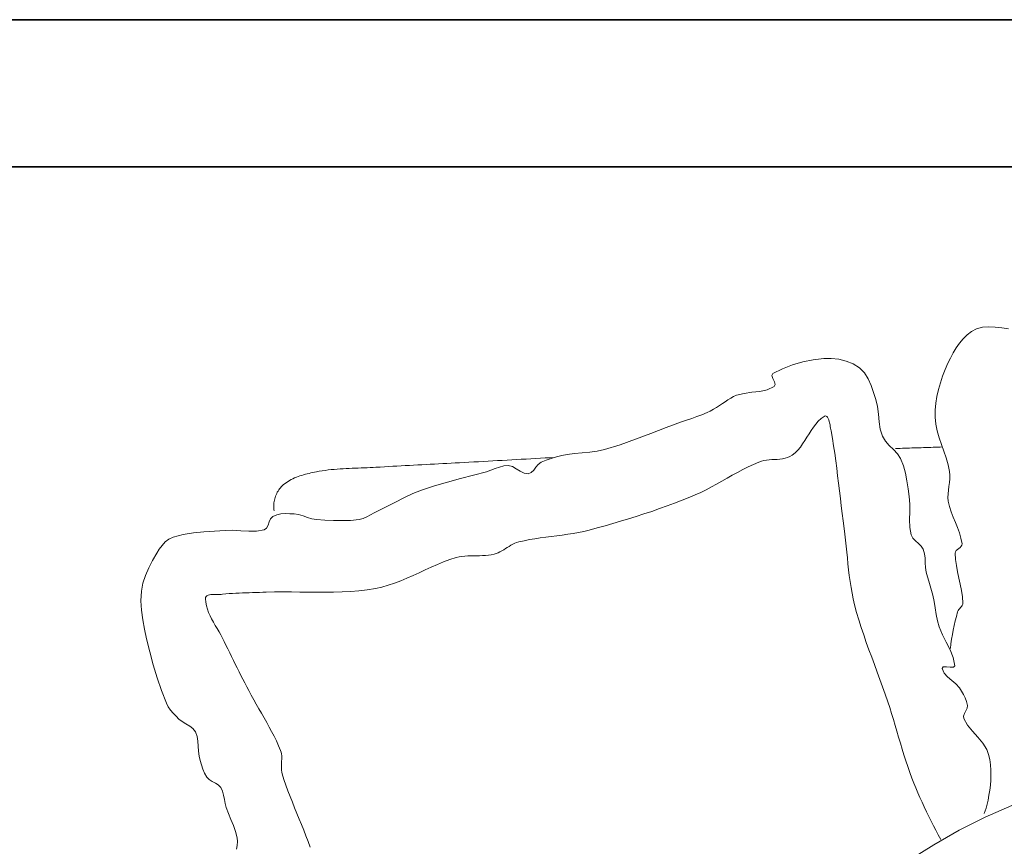
# Model space of a CAD drawing. Units: inches. Extents: x -36302355 to 648, y -221479757 to 75.
# Tile 26 of 37: x 190 to 220, y -192 to -167. Entities that reach past the tile are written whole.
import ezdxf

# ---------------------------------------------------------------- set-up
doc = ezdxf.new("R2010")
doc.units = ezdxf.units.IN
doc.header["$MEASUREMENT"] = 0
doc.layers.add('A-FURN', color=8, linetype='Continuous', lineweight=13)
doc.layers.add('A-WALL', color=7, linetype='Continuous', lineweight=35)

# ---------------------------------------------------------------- blocks, each defined once
blk = doc.blocks.new('BED-DOUBLE')
for p, q in [((26.757, 79.348), (26.607, 79.27)), ((26.943, 79.401), (26.757, 79.348)), ((27.135, 79.418), (26.943, 79.401)), ((27.332, 79.407), (27.135, 79.418)), ((27.532, 79.381), (27.332, 79.407)), ((27.733, 79.348), (27.532, 79.381)), ((26.347, 79.049), (26.235, 78.914)), ((26.471, 79.169), (26.347, 79.049)), ((26.607, 79.27), (26.471, 79.169)), ((26.134, 78.768), (26.042, 78.615)), ((26.235, 78.914), (26.134, 78.768)), ((21.435, 78.344), (21.756, 78.407)), ((21.756, 78.407), (22.08, 78.443)), ((22.08, 78.443), (22.309, 78.445)), ((22.309, 78.445), (22.541, 78.42)), ((22.541, 78.42), (22.768, 78.366)), ((25.959, 78.459), (25.883, 78.303)), ((26.042, 78.615), (25.959, 78.459)), ((20.524, 77.986), (20.815, 78.133)), ((20.815, 78.133), (21.12, 78.252)), ((21.12, 78.252), (21.435, 78.344)), ((22.768, 78.366), (22.981, 78.28)), ((22.981, 78.28), (23.172, 78.159)), ((23.172, 78.159), (23.323, 78.006)), ((25.797, 78.108), (25.719, 77.908)), ((25.883, 78.303), (25.797, 78.108)), ((20.495, 77.926), (20.524, 77.986)), ((20.521, 77.836), (20.495, 77.926)), ((20.567, 77.736), (20.521, 77.836)), ((23.323, 78.006), (23.44, 77.822)), ((23.44, 77.822), (23.532, 77.618)), ((25.719, 77.908), (25.65, 77.704)), ((20.119, 77.44), (20.35, 77.491)), ((20.35, 77.491), (20.565, 77.584)), ((20.565, 77.584), (20.594, 77.646)), ((20.594, 77.646), (20.567, 77.736)), ((23.532, 77.618), (23.607, 77.405)), ((25.593, 77.496), (25.546, 77.286)), ((25.65, 77.704), (25.593, 77.496)), ((19.065, 77.119), (19.147, 77.177)), ((19.147, 77.177), (19.23, 77.234)), ((19.23, 77.234), (19.317, 77.284)), ((19.317, 77.284), (19.408, 77.323)), ((19.408, 77.323), (19.64, 77.378)), ((19.64, 77.378), (19.88, 77.41)), ((19.88, 77.41), (20.119, 77.44)), ((23.607, 77.405), (23.677, 77.194)), ((23.677, 77.194), (23.73, 76.972)), ((25.546, 77.286), (25.513, 77.074)), ((18.605, 76.837), (18.7, 76.891)), ((18.7, 76.891), (18.794, 76.949)), ((18.794, 76.949), (18.887, 77.007)), ((18.887, 77.007), (18.98, 77.065)), ((18.98, 77.065), (19.065, 77.119)), ((23.73, 76.972), (23.756, 76.743)), ((25.513, 77.074), (25.494, 76.862)), ((17.88, 76.561), (18.038, 76.614)), ((18.038, 76.614), (18.196, 76.668)), ((18.196, 76.668), (18.352, 76.726)), ((18.352, 76.726), (18.506, 76.789)), ((18.506, 76.789), (18.605, 76.837)), ((21.911, 76.527), (21.997, 76.607)), ((21.997, 76.607), (22.092, 76.675)), ((22.092, 76.675), (22.122, 76.687)), ((22.122, 76.687), (22.15, 76.685)), ((22.15, 76.685), (22.174, 76.67)), ((22.174, 76.67), (22.196, 76.645)), ((22.196, 76.645), (22.215, 76.61)), ((22.215, 76.61), (22.232, 76.569)), ((22.232, 76.569), (22.247, 76.522)), ((23.756, 76.743), (23.776, 76.512)), ((25.494, 76.862), (25.489, 76.649)), ((25.489, 76.649), (25.507, 76.436)), ((16.786, 76.152), (17.253, 76.332)), ((17.253, 76.332), (17.722, 76.507)), ((17.722, 76.507), (17.88, 76.561)), ((21.693, 76.245), (21.761, 76.345)), ((21.761, 76.345), (21.833, 76.44)), ((21.833, 76.44), (21.911, 76.527)), ((22.247, 76.522), (22.26, 76.472)), ((22.26, 76.472), (22.271, 76.419)), ((22.271, 76.419), (22.281, 76.367)), ((22.281, 76.367), (22.29, 76.317)), ((22.29, 76.317), (22.297, 76.271)), ((22.297, 76.271), (22.304, 76.23)), ((23.776, 76.512), (23.809, 76.285)), ((23.809, 76.285), (23.875, 76.067)), ((25.507, 76.436), (25.55, 76.227)), ((15.847, 75.807), (16.318, 75.975)), ((16.318, 75.975), (16.786, 76.152)), ((21.5, 75.934), (21.565, 76.038)), ((21.565, 76.038), (21.628, 76.142)), ((21.628, 76.142), (21.693, 76.245)), ((22.304, 76.23), (22.343, 76.002)), ((22.343, 76.002), (22.38, 75.774)), ((23.875, 76.067), (23.965, 75.917)), ((25.55, 76.227), (25.61, 76.02)), ((25.61, 76.02), (25.681, 75.814)), ((15.37, 75.658), (15.847, 75.807)), ((21.288, 75.644), (21.364, 75.736)), ((21.364, 75.736), (21.434, 75.833)), ((21.434, 75.833), (21.5, 75.934)), ((22.38, 75.774), (22.414, 75.545)), ((23.965, 75.917), (24.086, 75.786)), ((24.086, 75.786), (24.218, 75.662)), ((24.218, 75.662), (24.341, 75.531)), ((24.272, 75.689), (24.344, 75.691)), ((24.344, 75.691), (24.416, 75.694)), ((24.416, 75.694), (24.488, 75.697)), ((24.488, 75.697), (24.56, 75.699)), ((24.56, 75.699), (24.632, 75.702)), ((24.632, 75.702), (24.704, 75.704)), ((24.704, 75.704), (24.776, 75.707)), ((24.776, 75.707), (24.848, 75.709)), ((24.848, 75.709), (24.92, 75.712)), ((24.92, 75.712), (24.992, 75.714)), ((24.992, 75.714), (25.064, 75.717)), ((25.064, 75.717), (25.136, 75.719)), ((25.136, 75.719), (25.208, 75.722)), ((25.208, 75.722), (25.28, 75.724)), ((25.28, 75.724), (25.353, 75.727)), ((25.353, 75.727), (25.425, 75.729)), ((25.425, 75.729), (25.497, 75.732)), ((25.497, 75.732), (25.569, 75.734)), ((25.569, 75.734), (25.641, 75.737)), ((25.641, 75.737), (25.713, 75.74)), ((25.681, 75.814), (25.756, 75.609)), ((12.675, 75.353), (12.821, 75.362)), ((12.821, 75.362), (12.966, 75.37)), ((12.966, 75.37), (13.112, 75.378)), ((13.112, 75.378), (13.258, 75.386)), ((13.258, 75.386), (13.403, 75.395)), ((13.403, 75.395), (13.549, 75.403)), ((13.549, 75.403), (13.694, 75.411)), ((13.578, 75.336), (13.736, 75.39)), ((13.694, 75.411), (13.84, 75.419)), ((13.736, 75.39), (13.898, 75.435)), ((13.898, 75.435), (14.062, 75.473)), ((14.062, 75.473), (14.226, 75.506)), ((14.226, 75.506), (14.454, 75.541)), ((14.454, 75.541), (14.685, 75.562)), ((14.685, 75.562), (14.916, 75.581)), ((14.916, 75.581), (15.145, 75.609)), ((15.145, 75.609), (15.37, 75.658)), ((20.576, 75.355), (20.658, 75.36)), ((20.658, 75.36), (20.74, 75.367)), ((20.74, 75.367), (20.82, 75.378)), ((20.82, 75.378), (20.898, 75.394)), ((20.898, 75.394), (20.973, 75.417)), ((20.973, 75.417), (21.045, 75.447)), ((21.045, 75.447), (21.112, 75.488)), ((21.112, 75.488), (21.205, 75.561)), ((21.205, 75.561), (21.288, 75.644)), ((22.414, 75.545), (22.446, 75.315)), ((24.341, 75.531), (24.434, 75.383)), ((24.434, 75.383), (24.518, 75.161)), ((25.756, 75.609), (25.827, 75.404)), ((25.827, 75.404), (25.889, 75.196)), ((7.089, 75.053), (7.18, 75.06)), ((7.18, 75.06), (7.272, 75.067)), ((7.272, 75.067), (7.363, 75.072)), ((7.363, 75.072), (7.455, 75.077)), ((7.455, 75.077), (7.547, 75.081)), ((7.547, 75.081), (7.639, 75.085)), ((7.639, 75.085), (7.73, 75.088)), ((7.73, 75.088), (7.822, 75.091)), ((7.822, 75.091), (7.914, 75.095)), ((7.914, 75.095), (8.006, 75.098)), ((8.006, 75.098), (8.098, 75.102)), ((8.098, 75.102), (8.189, 75.106)), ((8.189, 75.106), (8.281, 75.11)), ((8.281, 75.11), (8.372, 75.116)), ((8.372, 75.116), (8.5, 75.124)), ((8.5, 75.124), (8.628, 75.131)), ((8.628, 75.131), (8.756, 75.139)), ((8.756, 75.139), (8.883, 75.146)), ((8.883, 75.146), (9.011, 75.154)), ((9.011, 75.154), (9.139, 75.161)), ((9.139, 75.161), (9.267, 75.168)), ((9.267, 75.168), (9.394, 75.175)), ((9.394, 75.175), (9.522, 75.181)), ((9.522, 75.181), (9.65, 75.188)), ((9.65, 75.188), (9.778, 75.195)), ((9.778, 75.195), (9.906, 75.201)), ((9.906, 75.201), (10.033, 75.208)), ((10.033, 75.208), (10.161, 75.215)), ((10.161, 75.215), (10.289, 75.221)), ((10.289, 75.221), (10.417, 75.228)), ((10.417, 75.228), (10.545, 75.235)), ((10.545, 75.235), (10.672, 75.242)), ((10.672, 75.242), (10.8, 75.248)), ((10.8, 75.248), (10.928, 75.255)), ((10.928, 75.255), (11.074, 75.264)), ((11.074, 75.264), (11.219, 75.272)), ((11.219, 75.272), (11.365, 75.28)), ((11.365, 75.28), (11.511, 75.288)), ((11.511, 75.288), (11.656, 75.296)), ((11.656, 75.296), (11.802, 75.304)), ((11.802, 75.304), (11.947, 75.312)), ((11.888, 75.025), (12.019, 75.077)), ((11.947, 75.312), (12.093, 75.321)), ((12.019, 75.077), (12.151, 75.125)), ((12.093, 75.321), (12.238, 75.329)), ((12.151, 75.125), (12.284, 75.159)), ((12.238, 75.329), (12.384, 75.337)), ((12.284, 75.159), (12.419, 75.168)), ((12.384, 75.337), (12.53, 75.345)), ((12.419, 75.168), (12.546, 75.136)), ((12.53, 75.345), (12.675, 75.353)), ((12.546, 75.136), (12.666, 75.069)), ((12.666, 75.069), (12.784, 74.994)), ((13.199, 75.028), (13.268, 75.118)), ((13.268, 75.118), (13.34, 75.205)), ((13.34, 75.205), (13.425, 75.27)), ((13.425, 75.27), (13.578, 75.336)), ((19.599, 75.045), (19.762, 75.127)), ((19.762, 75.127), (19.927, 75.205)), ((19.927, 75.205), (20.094, 75.277)), ((20.094, 75.277), (20.17, 75.303)), ((20.17, 75.303), (20.248, 75.322)), ((20.248, 75.322), (20.328, 75.335)), ((20.328, 75.335), (20.41, 75.344)), ((20.41, 75.344), (20.493, 75.35)), ((20.493, 75.35), (20.576, 75.355)), ((22.446, 75.315), (22.476, 75.086)), ((22.476, 75.086), (22.505, 74.856)), ((24.518, 75.161), (24.58, 74.932)), ((25.889, 75.196), (25.933, 74.985)), ((5.779, 74.741), (5.83, 74.766)), ((5.83, 74.766), (5.882, 74.79)), ((5.882, 74.79), (5.935, 74.812)), ((5.935, 74.812), (5.988, 74.832)), ((5.988, 74.832), (6.043, 74.852)), ((6.043, 74.852), (6.098, 74.869)), ((6.098, 74.869), (6.153, 74.886)), ((6.153, 74.886), (6.209, 74.902)), ((6.209, 74.902), (6.265, 74.916)), ((6.265, 74.916), (6.322, 74.93)), ((6.322, 74.93), (6.378, 74.943)), ((6.378, 74.943), (6.434, 74.955)), ((6.434, 74.955), (6.49, 74.967)), ((6.49, 74.967), (6.546, 74.978)), ((6.546, 74.978), (6.636, 74.995)), ((6.636, 74.995), (6.726, 75.01)), ((6.726, 75.01), (6.816, 75.023)), ((6.816, 75.023), (6.907, 75.034)), ((6.907, 75.034), (6.998, 75.044)), ((6.998, 75.044), (7.089, 75.053)), ((10.558, 74.665), (10.958, 74.77)), ((10.958, 74.77), (11.358, 74.873)), ((11.358, 74.873), (11.757, 74.981)), ((11.757, 74.981), (11.888, 75.025)), ((12.784, 74.994), (12.904, 74.935)), ((12.904, 74.935), (13.03, 74.919)), ((13.03, 74.919), (13.123, 74.955)), ((13.123, 74.955), (13.199, 75.028)), ((18.958, 74.692), (19.118, 74.782)), ((19.118, 74.782), (19.277, 74.871)), ((19.277, 74.871), (19.437, 74.959)), ((19.437, 74.959), (19.599, 75.045)), ((22.505, 74.856), (22.533, 74.626)), ((24.58, 74.932), (24.626, 74.698)), ((25.939, 74.761), (25.927, 74.648)), ((25.933, 74.985), (25.942, 74.873)), ((25.942, 74.873), (25.939, 74.761)), ((5.395, 74.425), (5.419, 74.459)), ((5.419, 74.459), (5.445, 74.491)), ((5.445, 74.491), (5.472, 74.521)), ((5.472, 74.521), (5.501, 74.549)), ((5.501, 74.549), (5.544, 74.587)), ((5.544, 74.587), (5.588, 74.622)), ((5.588, 74.622), (5.633, 74.654)), ((5.633, 74.654), (5.68, 74.685)), ((5.68, 74.685), (5.729, 74.714)), ((5.729, 74.714), (5.779, 74.741)), ((9.77, 74.421), (10.161, 74.551)), ((10.161, 74.551), (10.558, 74.665)), ((18.476, 74.431), (18.638, 74.516)), ((18.638, 74.516), (18.798, 74.603)), ((18.798, 74.603), (18.958, 74.692)), ((22.533, 74.626), (22.56, 74.396)), ((24.626, 74.698), (24.663, 74.462)), ((24.663, 74.462), (24.695, 74.226)), ((25.911, 74.534), (25.895, 74.421)), ((25.927, 74.648), (25.911, 74.534)), ((5.262, 74.114), (5.273, 74.156)), ((5.273, 74.156), (5.285, 74.197)), ((5.285, 74.197), (5.299, 74.237)), ((5.299, 74.237), (5.314, 74.277)), ((5.314, 74.277), (5.332, 74.316)), ((5.332, 74.316), (5.351, 74.353)), ((5.351, 74.353), (5.372, 74.39)), ((5.372, 74.39), (5.395, 74.425)), ((8.965, 74.05), (9.228, 74.184)), ((9.228, 74.184), (9.496, 74.31)), ((9.496, 74.31), (9.77, 74.421)), ((17.748, 74.11), (17.98, 74.202)), ((17.98, 74.202), (18.148, 74.273)), ((18.148, 74.273), (18.313, 74.35)), ((18.313, 74.35), (18.476, 74.431)), ((22.56, 74.396), (22.588, 74.166)), ((22.588, 74.166), (22.615, 73.936)), ((24.695, 74.226), (24.712, 73.99)), ((25.884, 74.308), (25.882, 74.196)), ((25.882, 74.196), (25.893, 74.084)), ((25.895, 74.421), (25.884, 74.308)), ((5.242, 73.946), (5.244, 73.988)), ((5.242, 73.905), (5.242, 73.946)), ((5.245, 73.864), (5.242, 73.905)), ((5.244, 73.988), (5.248, 74.03)), ((5.249, 73.823), (5.245, 73.864)), ((5.248, 74.03), (5.254, 74.072)), ((5.254, 74.072), (5.262, 74.114)), ((8.436, 73.783), (8.701, 73.914)), ((8.701, 73.914), (8.965, 74.05)), ((16.812, 73.769), (17.047, 73.851)), ((17.047, 73.851), (17.282, 73.935)), ((17.282, 73.935), (17.515, 74.022)), ((17.515, 74.022), (17.748, 74.11)), ((22.615, 73.936), (22.643, 73.706)), ((24.712, 73.99), (24.71, 73.753)), ((25.893, 74.084), (25.931, 73.917)), ((25.931, 73.917), (25.983, 73.753)), ((5.146, 73.544), (5.214, 73.612)), ((5.214, 73.612), (5.335, 73.661)), ((5.256, 73.784), (5.249, 73.823)), ((5.335, 73.661), (5.463, 73.688)), ((5.463, 73.688), (5.596, 73.698)), ((5.596, 73.698), (5.731, 73.697)), ((5.731, 73.697), (5.863, 73.69)), ((5.863, 73.69), (6.003, 73.668)), ((6.003, 73.668), (6.139, 73.629)), ((6.139, 73.629), (6.275, 73.584)), ((6.275, 73.584), (6.411, 73.544)), ((7.853, 73.521), (7.976, 73.551)), ((7.976, 73.551), (8.094, 73.6)), ((8.094, 73.6), (8.208, 73.66)), ((8.208, 73.66), (8.321, 73.724)), ((8.321, 73.724), (8.436, 73.783)), ((16.101, 73.538), (16.338, 73.612)), ((16.338, 73.612), (16.575, 73.69)), ((16.575, 73.69), (16.812, 73.769)), ((22.643, 73.706), (22.672, 73.476)), ((24.71, 73.753), (24.706, 73.515)), ((25.983, 73.753), (26.044, 73.592)), ((26.044, 73.592), (26.109, 73.431)), ((4.945, 73.202), (5.019, 73.255)), ((5.019, 73.255), (5.066, 73.344)), ((5.066, 73.344), (5.102, 73.448)), ((5.102, 73.448), (5.146, 73.544)), ((6.411, 73.544), (6.55, 73.52)), ((6.55, 73.52), (6.81, 73.5)), ((6.81, 73.5), (7.072, 73.487)), ((7.072, 73.487), (7.333, 73.484)), ((7.333, 73.484), (7.594, 73.494)), ((7.594, 73.494), (7.853, 73.521)), ((14.902, 73.196), (15.143, 73.26)), ((15.143, 73.26), (15.383, 73.326)), ((15.383, 73.326), (15.623, 73.395)), ((15.623, 73.395), (15.862, 73.465)), ((15.862, 73.465), (16.101, 73.538)), ((22.672, 73.476), (22.703, 73.247)), ((24.706, 73.515), (24.715, 73.279)), ((24.715, 73.279), (24.755, 73.049)), ((26.109, 73.431), (26.174, 73.271)), ((26.174, 73.271), (26.233, 73.109)), ((2.033, 72.919), (2.158, 72.979)), ((2.158, 72.979), (2.468, 73.062)), ((2.468, 73.062), (2.784, 73.114)), ((2.784, 73.114), (3.106, 73.145)), ((3.106, 73.145), (3.429, 73.167)), ((3.429, 73.167), (3.751, 73.188)), ((3.751, 73.188), (3.991, 73.191)), ((3.991, 73.191), (4.232, 73.175)), ((4.232, 73.175), (4.474, 73.159)), ((4.474, 73.159), (4.712, 73.161)), ((4.712, 73.161), (4.945, 73.202)), ((13.235, 72.933), (13.402, 72.958)), ((13.402, 72.958), (13.57, 72.981)), ((13.57, 72.981), (13.738, 73.003)), ((13.738, 73.003), (13.905, 73.023)), ((13.905, 73.023), (14.073, 73.045)), ((14.073, 73.045), (14.24, 73.068)), ((14.24, 73.068), (14.407, 73.094)), ((14.407, 73.094), (14.573, 73.123)), ((14.573, 73.123), (14.738, 73.157)), ((14.738, 73.157), (14.902, 73.196)), ((22.703, 73.247), (22.726, 73.067)), ((22.726, 73.067), (22.746, 72.887)), ((24.755, 73.049), (24.805, 72.949)), ((24.805, 72.949), (24.884, 72.864)), ((26.233, 73.109), (26.28, 72.944)), ((1.735, 72.608), (1.822, 72.725)), ((1.822, 72.725), (1.921, 72.832)), ((1.921, 72.832), (2.033, 72.919)), ((12.337, 72.628), (12.392, 72.663)), ((12.392, 72.663), (12.448, 72.698)), ((12.448, 72.698), (12.504, 72.732)), ((12.504, 72.732), (12.56, 72.763)), ((12.56, 72.763), (12.619, 72.791)), ((12.619, 72.791), (12.678, 72.815)), ((12.678, 72.815), (12.74, 72.833)), ((12.74, 72.833), (12.904, 72.872)), ((12.904, 72.872), (13.069, 72.905)), ((13.069, 72.905), (13.235, 72.933)), ((22.746, 72.887), (22.765, 72.706)), ((22.765, 72.706), (22.784, 72.525)), ((24.884, 72.864), (24.976, 72.786)), ((24.976, 72.786), (25.061, 72.704)), ((25.061, 72.704), (25.122, 72.608)), ((26.252, 72.666), (26.212, 72.634)), ((26.286, 72.699), (26.252, 72.666)), ((26.28, 72.944), (26.312, 72.776)), ((26.308, 72.735), (26.286, 72.699)), ((26.312, 72.776), (26.308, 72.735)), ((1.534, 72.267), (1.658, 72.486)), ((1.658, 72.486), (1.735, 72.608)), ((10.634, 72.291), (10.828, 72.353)), ((10.828, 72.353), (10.915, 72.374)), ((10.915, 72.374), (11.003, 72.389)), ((11.003, 72.389), (11.092, 72.399)), ((11.092, 72.399), (11.181, 72.406)), ((11.181, 72.406), (11.271, 72.409)), ((11.271, 72.409), (11.362, 72.41)), ((11.362, 72.41), (11.453, 72.411)), ((11.453, 72.411), (11.543, 72.412)), ((11.543, 72.412), (11.634, 72.414)), ((11.634, 72.414), (11.723, 72.419)), ((11.723, 72.419), (11.813, 72.427)), ((11.813, 72.427), (11.901, 72.44)), ((11.901, 72.44), (11.989, 72.458)), ((11.989, 72.458), (12.05, 72.477)), ((12.05, 72.477), (12.11, 72.501)), ((12.11, 72.501), (12.168, 72.529)), ((12.168, 72.529), (12.225, 72.56)), ((12.225, 72.56), (12.281, 72.593)), ((12.281, 72.593), (12.337, 72.628)), ((22.784, 72.525), (22.802, 72.344)), ((22.802, 72.344), (22.82, 72.164)), ((25.122, 72.608), (25.161, 72.474)), ((25.161, 72.474), (25.18, 72.335)), ((26.111, 72.533), (26.102, 72.492)), ((26.102, 72.492), (26.114, 72.299)), ((26.136, 72.57), (26.111, 72.533)), ((26.172, 72.603), (26.136, 72.57)), ((26.212, 72.634), (26.172, 72.603)), ((1.316, 71.81), (1.417, 72.042)), ((1.417, 72.042), (1.534, 72.267)), ((9.878, 71.977), (10.065, 72.062)), ((10.065, 72.062), (10.253, 72.144)), ((10.253, 72.144), (10.442, 72.221)), ((10.442, 72.221), (10.634, 72.291)), ((22.82, 72.164), (22.84, 71.983)), ((25.18, 72.335), (25.188, 72.193)), ((25.188, 72.193), (25.197, 72.051)), ((25.197, 72.051), (25.217, 71.912)), ((26.114, 72.299), (26.14, 72.108)), ((26.14, 72.108), (26.176, 71.917)), ((1.238, 71.572), (1.316, 71.81)), ((9.318, 71.722), (9.506, 71.805)), ((9.506, 71.805), (9.692, 71.891)), ((9.692, 71.891), (9.878, 71.977)), ((22.84, 71.983), (22.862, 71.803)), ((22.862, 71.803), (22.886, 71.623)), ((25.217, 71.912), (25.252, 71.769)), ((25.252, 71.769), (25.294, 71.628)), ((26.176, 71.917), (26.217, 71.727)), ((1.19, 71.327), (1.238, 71.572)), ((8.354, 71.408), (8.553, 71.451)), ((8.553, 71.451), (8.748, 71.506)), ((8.748, 71.506), (8.94, 71.57)), ((8.94, 71.57), (9.13, 71.643)), ((9.13, 71.643), (9.318, 71.722)), ((22.886, 71.623), (22.914, 71.444)), ((22.914, 71.444), (22.945, 71.266)), ((25.294, 71.628), (25.339, 71.487)), ((25.339, 71.487), (25.382, 71.346)), ((26.217, 71.727), (26.258, 71.537)), ((26.258, 71.537), (26.296, 71.346)), ((1.175, 71.036), (1.19, 71.327)), ((3.155, 71.133), (3.171, 71.163)), ((3.171, 71.163), (3.197, 71.186)), ((3.197, 71.186), (3.231, 71.202)), ((3.231, 71.202), (3.271, 71.214)), ((3.271, 71.214), (3.318, 71.222)), ((3.318, 71.222), (3.368, 71.226)), ((3.368, 71.226), (3.421, 71.228)), ((3.421, 71.228), (3.475, 71.228)), ((3.475, 71.228), (3.529, 71.228)), ((3.529, 71.228), (3.581, 71.228)), ((3.581, 71.228), (3.63, 71.229)), ((3.63, 71.229), (3.674, 71.232)), ((3.674, 71.232), (3.776, 71.243)), ((3.776, 71.243), (3.879, 71.251)), ((3.879, 71.251), (3.981, 71.258)), ((3.981, 71.258), (4.083, 71.264)), ((4.083, 71.264), (4.186, 71.27)), ((4.186, 71.27), (4.288, 71.274)), ((4.288, 71.274), (4.391, 71.277)), ((4.391, 71.277), (4.494, 71.281)), ((4.494, 71.281), (4.596, 71.283)), ((4.596, 71.283), (4.699, 71.286)), ((4.699, 71.286), (4.801, 71.289)), ((4.801, 71.289), (4.904, 71.292)), ((4.904, 71.292), (5.007, 71.296)), ((5.007, 71.296), (5.264, 71.303)), ((5.264, 71.303), (5.523, 71.305)), ((5.523, 71.305), (5.781, 71.304)), ((5.781, 71.304), (6.04, 71.301)), ((6.04, 71.301), (6.299, 71.297)), ((6.299, 71.297), (6.558, 71.294)), ((6.558, 71.294), (6.816, 71.293)), ((6.816, 71.293), (7.074, 71.296)), ((7.074, 71.296), (7.332, 71.303)), ((7.332, 71.303), (7.589, 71.317)), ((7.589, 71.317), (7.845, 71.338)), ((7.845, 71.338), (8.1, 71.368)), ((8.1, 71.368), (8.354, 71.408)), ((22.945, 71.266), (22.982, 71.089)), ((25.382, 71.346), (25.42, 71.204)), ((25.42, 71.204), (25.46, 71.009)), ((26.296, 71.346), (26.325, 71.155)), ((26.325, 71.155), (26.341, 70.962)), ((1.191, 70.743), (1.175, 71.036)), ((3.15, 71.095), (3.155, 71.133)), ((3.16, 70.987), (3.15, 71.095)), ((3.18, 70.881), (3.16, 70.987)), ((3.21, 70.777), (3.18, 70.881)), ((22.982, 71.089), (23.023, 70.912)), ((23.023, 70.912), (23.085, 70.679)), ((25.46, 71.009), (25.493, 70.813)), ((26.298, 70.858), (26.271, 70.827)), ((26.321, 70.891), (26.298, 70.858)), ((26.336, 70.925), (26.321, 70.891)), ((26.341, 70.962), (26.336, 70.925)), ((1.231, 70.451), (1.191, 70.743)), ((3.248, 70.675), (3.21, 70.777)), ((3.292, 70.575), (3.248, 70.675)), ((3.341, 70.476), (3.292, 70.575)), ((23.085, 70.679), (23.153, 70.448)), ((25.493, 70.813), (25.525, 70.617)), ((25.525, 70.617), (25.564, 70.423)), ((26.14, 70.556), (26.106, 70.417)), ((26.177, 70.695), (26.14, 70.556)), ((26.192, 70.731), (26.177, 70.695)), ((26.215, 70.764), (26.192, 70.731)), ((26.242, 70.796), (26.215, 70.764)), ((26.271, 70.827), (26.242, 70.796)), ((1.287, 70.16), (1.231, 70.451)), ((3.395, 70.377), (3.341, 70.476)), ((3.451, 70.28), (3.395, 70.377)), ((3.509, 70.182), (3.451, 70.28)), ((23.153, 70.448), (23.225, 70.218)), ((25.564, 70.423), (25.614, 70.231)), ((26.074, 70.278), (26.045, 70.138)), ((26.106, 70.417), (26.074, 70.278)), ((1.35, 69.873), (1.287, 70.16)), ((3.566, 70.085), (3.509, 70.182)), ((3.622, 69.988), (3.566, 70.085)), ((3.676, 69.89), (3.622, 69.988)), ((23.225, 70.218), (23.302, 69.989)), ((23.302, 69.989), (23.381, 69.761)), ((25.614, 70.231), (25.71, 69.993)), ((25.71, 69.993), (25.829, 69.762)), ((26.019, 69.997), (25.995, 69.856)), ((26.045, 70.138), (26.019, 69.997)), ((1.446, 69.472), (1.35, 69.873)), ((3.725, 69.791), (3.676, 69.89)), ((3.78, 69.675), (3.725, 69.791)), ((3.836, 69.558), (3.78, 69.675)), ((23.381, 69.761), (23.463, 69.534)), ((25.829, 69.762), (25.948, 69.531)), ((25.974, 69.714), (25.956, 69.572)), ((25.995, 69.856), (25.974, 69.714)), ((1.554, 69.073), (1.446, 69.472)), ((3.893, 69.442), (3.836, 69.558)), ((3.949, 69.326), (3.893, 69.442)), ((23.463, 69.534), (23.547, 69.307)), ((25.948, 69.531), (26.043, 69.295)), ((1.675, 68.678), (1.554, 69.073)), ((4.007, 69.21), (3.949, 69.326)), ((4.064, 69.095), (4.007, 69.21)), ((4.122, 68.979), (4.064, 69.095)), ((23.547, 69.307), (23.632, 69.08)), ((23.632, 69.08), (23.716, 68.854)), ((26.043, 69.295), (26.093, 69.048)), ((26.093, 69.048), (26.054, 69.001)), ((4.18, 68.864), (4.122, 68.979)), ((4.239, 68.749), (4.18, 68.864)), ((4.298, 68.634), (4.239, 68.749)), ((23.716, 68.854), (23.801, 68.627)), ((25.738, 69.008), (25.707, 68.962)), ((25.707, 68.962), (25.768, 68.822)), ((25.834, 69.01), (25.738, 69.008)), ((25.768, 68.822), (25.873, 68.704)), ((25.954, 68.998), (25.834, 69.01)), ((26.054, 69.001), (25.954, 68.998)), ((1.809, 68.288), (1.675, 68.678)), ((4.357, 68.519), (4.298, 68.634)), ((4.416, 68.404), (4.357, 68.519)), ((23.801, 68.627), (23.883, 68.4)), ((25.873, 68.704), (25.999, 68.598)), ((25.999, 68.598), (26.127, 68.49)), ((26.127, 68.49), (26.234, 68.369)), ((1.956, 67.902), (1.809, 68.288)), ((4.475, 68.289), (4.416, 68.404)), ((4.55, 68.148), (4.475, 68.289)), ((4.627, 68.007), (4.55, 68.148)), ((23.883, 68.4), (23.964, 68.172)), ((23.964, 68.172), (24.041, 67.944)), ((26.234, 68.369), (26.299, 68.27)), ((26.299, 68.27), (26.36, 68.166)), ((26.36, 68.166), (26.413, 68.059)), ((2.012, 67.792), (1.956, 67.902)), ((4.705, 67.868), (4.627, 68.007)), ((4.785, 67.729), (4.705, 67.868)), ((24.041, 67.944), (24.1, 67.764)), ((26.413, 68.059), (26.454, 67.948)), ((26.454, 67.948), (26.479, 67.833)), ((26.479, 67.833), (26.469, 67.749)), ((2.082, 67.69), (2.012, 67.792)), ((2.164, 67.594), (2.082, 67.69)), ((2.251, 67.503), (2.164, 67.594)), ((4.865, 67.59), (4.785, 67.729)), ((4.945, 67.451), (4.865, 67.59)), ((24.1, 67.764), (24.156, 67.584)), ((24.156, 67.584), (24.211, 67.403)), ((26.386, 67.585), (26.357, 67.505)), ((26.431, 67.667), (26.386, 67.585)), ((26.469, 67.749), (26.431, 67.667)), ((2.34, 67.415), (2.251, 67.503)), ((2.441, 67.335), (2.34, 67.415)), ((2.555, 67.267), (2.441, 67.335)), ((2.668, 67.2), (2.555, 67.267)), ((5.025, 67.311), (4.945, 67.451)), ((5.102, 67.171), (5.025, 67.311)), ((24.211, 67.403), (24.264, 67.222)), ((24.264, 67.222), (24.318, 67.041)), ((26.357, 67.505), (26.365, 67.427)), ((26.365, 67.427), (26.483, 67.224)), ((26.483, 67.224), (26.632, 67.041)), ((2.769, 67.123), (2.668, 67.2)), ((2.846, 67.024), (2.769, 67.123)), ((2.898, 66.886), (2.846, 67.024)), ((5.178, 67.03), (5.102, 67.171)), ((5.252, 66.888), (5.178, 67.03)), ((24.318, 67.041), (24.371, 66.86)), ((26.632, 67.041), (26.794, 66.864)), ((2.92, 66.738), (2.898, 66.886)), ((2.927, 66.585), (2.92, 66.738)), ((5.322, 66.745), (5.252, 66.888)), ((5.388, 66.599), (5.322, 66.745)), ((24.371, 66.86), (24.424, 66.679)), ((24.424, 66.679), (24.479, 66.498)), ((26.794, 66.864), (26.947, 66.682)), ((26.947, 66.682), (27.07, 66.482)), ((2.934, 66.432), (2.927, 66.585)), ((2.957, 66.283), (2.934, 66.432)), ((5.45, 66.452), (5.388, 66.599)), ((5.467, 66.4), (5.45, 66.452)), ((5.478, 66.347), (5.467, 66.4)), ((5.485, 66.293), (5.478, 66.347)), ((24.479, 66.498), (24.534, 66.317)), ((24.534, 66.317), (24.592, 66.138)), ((27.07, 66.482), (27.127, 66.334)), ((27.127, 66.334), (27.163, 66.178)), ((2.99, 66.148), (2.957, 66.283)), ((3.026, 66.014), (2.99, 66.148)), ((3.068, 65.882), (3.026, 66.014)), ((5.474, 65.958), (5.476, 66.014)), ((5.476, 66.014), (5.48, 66.07)), ((5.48, 66.07), (5.483, 66.126)), ((5.483, 66.126), (5.486, 66.183)), ((5.487, 66.238), (5.485, 66.293)), ((5.486, 66.183), (5.487, 66.238)), ((24.592, 66.138), (24.652, 65.959)), ((27.163, 66.178), (27.184, 66.017)), ((27.184, 66.017), (27.194, 65.855)), ((3.122, 65.755), (3.068, 65.882)), ((3.19, 65.637), (3.122, 65.755)), ((5.474, 65.902), (5.474, 65.958)), ((5.478, 65.847), (5.474, 65.902)), ((5.486, 65.793), (5.478, 65.847)), ((5.499, 65.74), (5.486, 65.793)), ((5.555, 65.564), (5.499, 65.74)), ((24.652, 65.959), (24.715, 65.781)), ((24.715, 65.781), (24.781, 65.604)), ((27.194, 65.855), (27.198, 65.694)), ((3.264, 65.562), (3.19, 65.637)), ((3.356, 65.506), (3.264, 65.562)), ((3.454, 65.455), (3.356, 65.506)), ((3.545, 65.398), (3.454, 65.455)), ((5.615, 65.389), (5.555, 65.564)), ((24.781, 65.604), (24.839, 65.456)), ((24.839, 65.456), (24.899, 65.309)), ((27.195, 65.541), (27.182, 65.388)), ((27.198, 65.694), (27.195, 65.541)), ((3.617, 65.322), (3.545, 65.398)), ((3.672, 65.208), (3.617, 65.322)), ((3.707, 65.086), (3.672, 65.208)), ((5.678, 65.215), (5.615, 65.389)), ((5.744, 65.043), (5.678, 65.215)), ((24.899, 65.309), (24.96, 65.162)), ((24.96, 65.162), (25.023, 65.015)), ((27.161, 65.236), (27.135, 65.084)), ((27.182, 65.388), (27.161, 65.236)), ((3.731, 64.958), (3.707, 65.086)), ((3.755, 64.83), (3.731, 64.958)), ((3.787, 64.705), (3.755, 64.83)), ((5.812, 64.871), (5.744, 65.043)), ((5.881, 64.699), (5.812, 64.871)), ((25.023, 65.015), (25.088, 64.87)), ((25.088, 64.87), (25.154, 64.725)), ((27.092, 64.849), (27.072, 64.767)), ((27.108, 64.932), (27.092, 64.849)), ((27.135, 65.084), (27.108, 64.932)), ((3.854, 64.521), (3.787, 64.705)), ((3.93, 64.339), (3.854, 64.521)), ((5.951, 64.528), (5.881, 64.699)), ((6.021, 64.357), (5.951, 64.528)), ((25.154, 64.725), (25.222, 64.581)), ((25.222, 64.581), (25.292, 64.438)), ((27.023, 64.605), (26.994, 64.526)), ((27.839, 64.768), (27.022, 64.416)), ((27.05, 64.686), (27.023, 64.605)), ((27.072, 64.767), (27.05, 64.686)), ((4.005, 64.157), (3.93, 64.339)), ((6.092, 64.186), (6.021, 64.357)), ((25.292, 64.438), (25.363, 64.295)), ((25.363, 64.295), (25.436, 64.153)), ((27.022, 64.416), (26.225, 64.013)), ((4.071, 63.972), (4.005, 64.157)), ((4.119, 63.783), (4.071, 63.972)), ((6.161, 64.014), (6.092, 64.186)), ((6.229, 63.842), (6.161, 64.014)), ((25.436, 64.153), (25.511, 64.013)), ((26.225, 64.013), (25.45, 63.569)), ((25.511, 64.013), (25.586, 63.873)), ((4.117, 63.548), (4.128, 63.666)), ((4.128, 63.666), (4.119, 63.783)), ((6.296, 63.67), (6.229, 63.842)), ((6.36, 63.496), (6.296, 63.67)), ((25.586, 63.873), (25.664, 63.734)), ((4.097, 63.43), (4.117, 63.548)), ((25.45, 63.569), (24.695, 63.097))]:
    blk.add_line(p, q)

msp = doc.modelspace()

# ---------------------------------------------------------------- linework, layer by layer
at = {"layer": 'A-WALL'}
for p, q in [((145.197, -167.019), (323.197, -167.019)), ((154.197, -171.519), (314.197, -171.519))]:
    msp.add_line(p, q, dxfattribs=at)

# ---------------------------------------------------------------- block references
at = {"layer": 'A-FURN'}
msp.add_blockref('BED-DOUBLE', (192.212, -255.828), dxfattribs=at)

doc.saveas('drawing.dxf')
